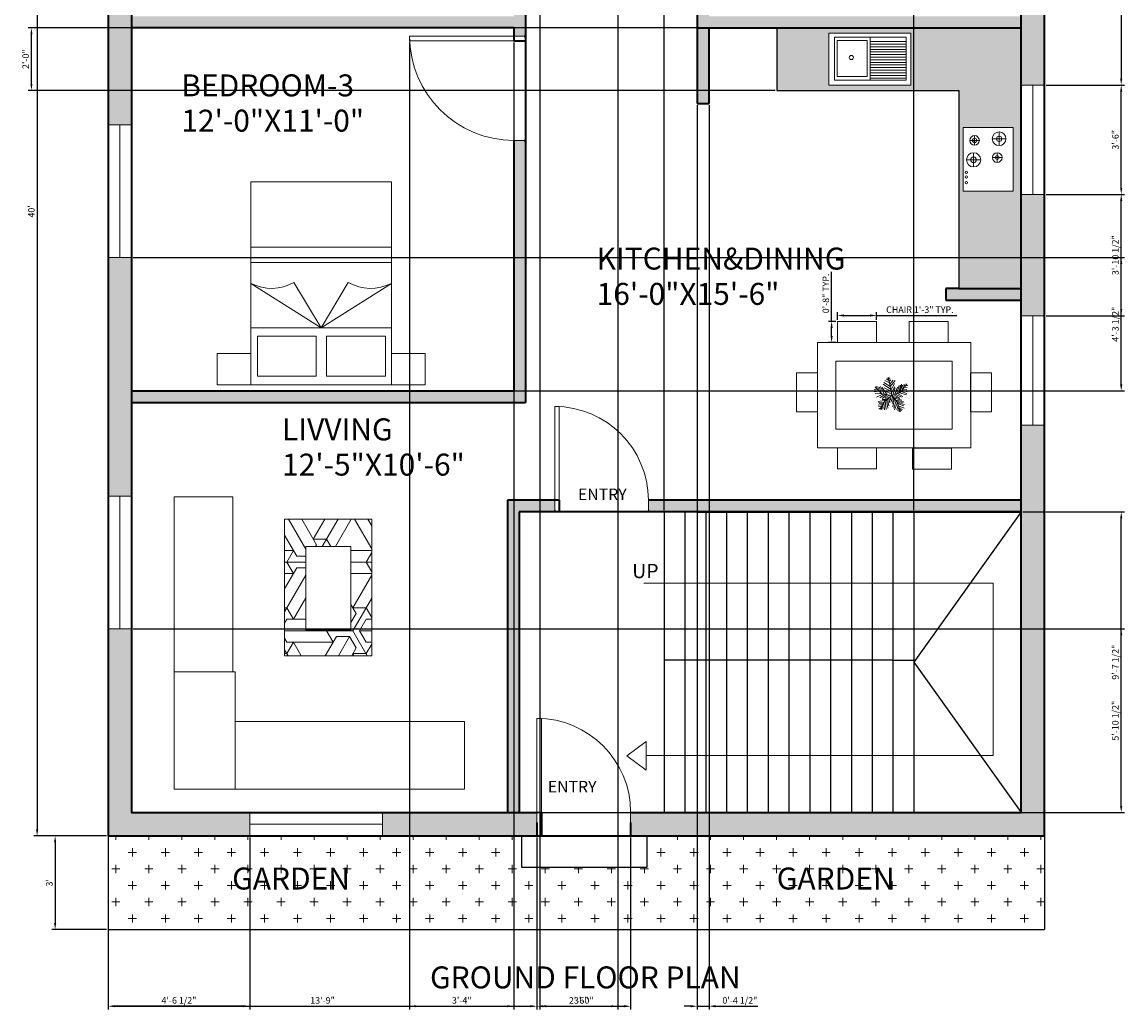
# Model space of a CAD drawing. Units: inches. Extents: x 10 to 434, y 91 to 681.
# Tile 1 of 2: x 10 to 434, y 91 to 471. Entities that reach past the tile are written whole.
import ezdxf

# ---------------------------------------------------------------- set-up
doc = ezdxf.new("R2010")
doc.units = ezdxf.units.IN
for name, color, linetype, lineweight in [('A-ANNO-DIMS', 2, 'Continuous', 18), ('A-ANNO-SYMB', 2, 'Continuous', 18), ('A-ANNO-TEXT', 7, 'Continuous', 18), ('A-AREA-IDEN', 7, 'Continuous', 18), ('A-DOOR', 4, 'Continuous', 18), ('A-EQPM', 8, 'Continuous', 18), ('A-FLOR-CASE', 8, 'Continuous', 25), ('A-FLOR-CASE-PATT', 141, 'Continuous', 13), ('A-FLOR-FIXT', 9, 'Continuous', 18), ('A-FLOR-FIXT-PATT', 9, 'Continuous', 13), ('A-FLOR-STRS', 7, 'Continuous', 25), ('A-FURN', 8, 'Continuous', 18), ('A-FURN-PATT', 8, 'Continuous', 13), ('A-GLAZ', 4, 'Continuous', 18), ('A-WALL', 7, 'Continuous', 35), ('A-WALL-PATT', 251, 'Continuous', 13), ('L-PLNT', 3, 'Continuous', 18), ('L-PLNT-BEDS', 3, 'Continuous', 25), ('L-PLNT-PATT', 114, 'Continuous', 13)]:
    doc.layers.add(name, color=color, linetype=linetype, lineweight=lineweight)
doc.styles.get("Standard").update_dxf_attribs({"font": 'arial.ttf'})
doc.dimstyles.new('ISO-25', dxfattribs={"dimtxt": 2.5, "dimasz": 2.5, "dimexe": 1.25, "dimexo": 0.625, "dimtad": 1, "dimlunit": 3, "dimtxsty": 'Standard', "dimcen": 2.5, "dimadec": 0, "dimazin": 0, "dimtfac": 1, "dimtmove": 0, "dimatfit": 3, "dimfxl": 1, "dimarcsym": 0})

# ---------------------------------------------------------------- blocks, each defined once
blk = doc.blocks.new('*U2')
for p, q in [((0, 0), (0, -4)), ((36, 0), (36, -4))]:
    blk.add_line(p, q)
blk.add_lwpolyline([(0, 0), (0, 36), (1.75, 36), (1.75, 0)], close=True)
blk.add_arc((0, 0), 36, 0, 90)
blk = doc.blocks.new('*U5')
for p, q in [((0, 0), (0, -4)), ((-40, 0), (-40, -4))]:
    blk.add_line(p, q)
blk.add_lwpolyline([(0, 0), (0, 40), (-1.75, 40), (-1.75, 0)], close=True)
blk.add_arc((0, 0), 40, 90, 180)
blk = doc.blocks.new('*U9')
for p, q in [((-3.665, 19.273), (-27.574, 35.527)), ((-5.114, 28.097), (-24.676, 40.636)), ((-7.288, 39.707), (-21.778, 46.673)), ((-8.737, 47.138), (-17.069, 52.711)), ((-10.186, 53.64), (-13.084, 55.962)), ((0, 0), (-10.5, 57)), ((-9.099, 51.782), (-6.563, 55.962)), ((-7.65, 43.423), (-2.578, 49.46)), ((-5.839, 35.992), (4.667, 48.067)), ((-5.114, 27.632), (10.463, 46.673)), ((-2.941, 16.486), (8.652, 37.85)), ((27, 9), (48, 36)), ((27.127, 9.056), (31.112, 35.992)), ((44.153, 36.456), (45.239, 32.741)), ((-47.498, 19.737), (-55.83, 18.344)), ((-40.615, 13.7), (-55.105, 10.913)), ((-31.5, 4.5), (-52.5, 25.5)), ((-33.37, 6.269), (-52.207, 5.34)), ((-48.585, 21.131), (-49.309, 29.026)), ((-28.299, 3.483), (-47.86, -5.805)), ((-43.513, 28.561), (-42.427, 15.558)), ((-38.442, 26.239), (-34.819, 7.663)), ((-21.416, 3.018), (-38.079, -8.128)), ((-35.544, 28.097), (-24.314, 3.947)), ((0, 0), (-31.5, 4.5)), ((-14.533, 2.09), (-30.834, 25.31)), ((-15.982, 2.09), (-30.11, -9.521)), ((-24.314, 23.917), (-2.941, 13.7)), ((0, 0), (-22.5, -19.5)), ((-6.563, 1.161), (-21.416, -8.128)), ((-20.691, 13.7), (-1.129, 4.876)), ((-1.129, 6.734), (9.014, 26.704)), ((0, 0), (27, 9)), ((0, 0), (18, -22.5)), ((3.942, 1.625), (11.187, 24.381)), ((6.478, 1.625), (26.04, -8.592)), ((10.101, 3.483), (17.708, 26.239)), ((11.187, 3.483), (30.749, -5.805)), ((16.259, 5.805), (23.142, 31.348)), ((18.07, 5.805), (35.096, -3.483)), ((22.055, 7.198), (27.489, 32.277)), ((24.229, 7.663), (46.688, 1.625)), ((29.662, 12.307), (48.137, 6.269)), ((31.836, 30.883), (32.561, 16.486)), ((33.285, 16.486), (48.862, 10.913)), ((35.096, 32.741), (37.27, 22.524)), ((36.183, 19.737), (48.137, 17.88)), ((38.719, 34.134), (41.979, 28.561)), ((40.53, 25.775), (48.862, 24.846)), ((43.791, 29.954), (51.036, 30.883)), ((-17.431, -15.094), (-42.789, -18.809)), ((-28.299, -29.026), (-42.789, -31.348)), ((-24.314, -21.596), (-42.427, -22.06)), ((-30.834, -34.135), (-42.427, -35.528)), ((-26.849, -26.24), (-40.253, -25.775)), ((-22.5, -19.5), (-37.5, -45)), ((-15.257, -12.772), (-30.11, -12.772)), ((-29.023, -30.884), (-27.936, -43.887)), ((-25.038, -23.918), (-22.865, -45.281)), ((-20.691, -18.345), (-17.793, -44.352)), ((-6.563, -5.805), (-19.967, -9.985)), ((-17.069, -15.094), (-12.721, -40.172)), ((-13.446, -11.378), (-8.737, -32.741)), ((-9.461, -8.592), (-6.201, -23.453)), ((-4.752, -3.483), (-3.665, -14.629)), ((2.493, -3.019), (-1.491, -20.202)), ((1.769, -2.555), (24.229, -9.521)), ((5.029, -6.27), (2.131, -25.775)), ((9.014, -11.378), (3.58, -35.992)), ((14.085, -16.951), (6.478, -40.172)), ((7.565, -9.056), (32.198, -14.629)), ((18.07, -22.524), (8.289, -45.745)), ((12.274, -15.094), (36.907, -18.809)), ((20.244, -30.419), (15.897, -44.816)), ((16.259, -19.738), (36.183, -22.989)), ((18, -22.5), (27, -52.5)), ((18.433, -22.524), (40.53, -29.026)), ((19.157, -25.311), (38.719, -33.206)), ((21.331, -32.741), (39.081, -40.636)), ((-34.457, -39.708), (-40.978, -42.494)), ((-32.646, -36.921), (-31.921, -44.352)), ((22.78, -37.85), (19.519, -48.532)), ((22.78, -38.314), (34.372, -44.816)), ((24.591, -45.745), (23.142, -50.854)), ((24.591, -43.423), (30.749, -47.603)), ((26.764, -49.925), (28.213, -50.854))]:
    blk.add_line(p, q)
blk = doc.blocks.new('*U10')
for p, q in [((0, 0), (0, -4)), ((36, 0), (36, -4))]:
    blk.add_line(p, q)
blk.add_lwpolyline([(0, 0), (0, 36), (1.75, 36), (1.75, 0)], close=True)
blk.add_arc((0, 0), 36, 0, 90)
blk = doc.blocks.new('*D11')
at = {"layer": 'A-ANNO-DIMS', "color": 0, "lineweight": -2, "transparency": 16777216}
for p, q in [((42.44, 638.74), (14.54, 638.74)), ((15.79, 636.24), (15.79, 161.24)), ((42.44, 158.74), (14.54, 158.74))]:
    blk.add_line(p, q, dxfattribs=at)
at = {"layer": 'A-ANNO-DIMS', "color": 0, "transparency": 16777216}
for points in [[(15.37, 636.24), (16.21, 636.24), (15.79, 638.74)], [(15.37, 161.24), (16.21, 161.24), (15.79, 158.74)]]:
    blk.add_solid(points, dxfattribs=at)
at = {"layer": 'Defpoints', "color": 0, "transparency": 16777216}
for p in [(43.07, 638.74), (15.79, 158.74), (43.07, 158.74)]:
    blk.add_point(p, dxfattribs=at)
at = {"layer": 'A-ANNO-DIMS', "color": 0, "transparency": 16777216, "insert": (13.89, 398.74), "char_height": 2.5, "attachment_point": 5, "rotation": 90}
blk.add_mtext("40'", dxfattribs=at)
blk = doc.blocks.new('*D13')
at = {"layer": 'A-ANNO-DIMS', "color": 0, "lineweight": -2, "transparency": 16777216}
for p, q in [((42.44, 158.74), (21.47, 158.74)), ((22.72, 156.24), (22.72, 125.24)), ((42.44, 122.74), (21.47, 122.74))]:
    blk.add_line(p, q, dxfattribs=at)
at = {"layer": 'A-ANNO-DIMS', "color": 0, "transparency": 16777216}
for points in [[(22.3, 156.24), (23.13, 156.24), (22.72, 158.74)], [(22.3, 125.24), (23.13, 125.24), (22.72, 122.74)]]:
    blk.add_solid(points, dxfattribs=at)
at = {"layer": 'Defpoints', "color": 0, "transparency": 16777216}
for p in [(43.07, 158.74), (22.72, 122.74), (43.07, 122.74)]:
    blk.add_point(p, dxfattribs=at)
at = {"layer": 'A-ANNO-DIMS', "color": 0, "transparency": 16777216, "insert": (20.81, 140.74), "char_height": 2.5, "attachment_point": 5, "rotation": 90}
blk.add_mtext("3'", dxfattribs=at)
blk = doc.blocks.new('BED-DOUBLE-WITH-NIGHTSTANDS')
for p, q in [((40, 21.85), (13, 39)), ((40, 21.85), (29.54, 39.37)), ((40, 21.85), (50.46, 39.37)), ((40, 21.85), (67, 39)), ((67, 21.85), (13, 21.85)), ((38.13, 3.34), (38.13, 18.76)), ((42.13, 3.34), (42.13, 18.76)), ((0, 0), (0, 12)), ((0, 12), (13, 12)), ((68, 12), (67, 12)), ((80, 12), (68, 12)), ((80, 0), (80, 12)), ((1, 0), (0, 0)), ((13, 0), (1, 0)), ((68, 0), (80, 0))]:
    blk.add_line(p, q)
for points in [[(67, 78), (13, 78), (13, 0), (67, 0)], [(67, 46.98), (13, 46.98), (13, 52.9), (67, 52.9)], [(67, 0), (68, 0), (68, 0), (67, 0)]]:
    blk.add_lwpolyline(points, close=True)
for points in [[(38.13, 3.34), (15.5, 3.34), (15.5, 18.76), (38.13, 18.76)], [(42.13, 18.76), (64.76, 18.76), (64.76, 3.34), (42.13, 3.34)]]:
    blk.add_lwpolyline(points)
for centre, start, end in [((20.93, 54.43), 242.8058, 299.7512), ((59.07, 54.43), 240.2488, 297.1942)]:
    blk.add_arc(centre, 17.35, start, end)
blk = doc.blocks.new('DINING-CHAIR')
blk.add_lwpolyline([(0, 0), (15.04, 0), (15.04, 8.09), (0, 8.09)], close=True)
blk = doc.blocks.new('WINDOW-51IN')
for p, q in [((0, 9), (0, 0)), ((51, 4.5), (51, 9)), ((51, 9), (51, 0)), ((0, 0), (0, 4.5)), ((0, 4.5), (51, 4.5))]:
    blk.add_line(p, q)
blk = doc.blocks.new('*D18')
at = {"layer": 'A-ANNO-DIMS', "color": 0, "lineweight": -2, "transparency": 16777216}
for p, q in [((323.44, 357.1), (323.44, 359.98)), ((325.94, 358.73), (335.98, 358.73)), ((338.48, 357.1), (338.48, 359.98)), ((338.48, 358.73), (369.27, 358.73))]:
    blk.add_line(p, q, dxfattribs=at)
at = {"layer": 'A-ANNO-DIMS', "color": 0, "transparency": 16777216}
for points in [[(325.94, 359.15), (325.94, 358.31), (323.44, 358.73)], [(335.98, 359.15), (335.98, 358.31), (338.48, 358.73)]]:
    blk.add_solid(points, dxfattribs=at)
at = {"layer": 'Defpoints', "color": 0, "transparency": 16777216}
for p in [(323.44, 356.47), (338.48, 358.73), (338.48, 356.47)]:
    blk.add_point(p, dxfattribs=at)
at = {"layer": 'A-ANNO-DIMS', "color": 0, "transparency": 16777216, "insert": (355.13, 360.65), "char_height": 2.5, "attachment_point": 5}
blk.add_mtext('CHAIR 1\'-3" TYP.', dxfattribs=at)
blk = doc.blocks.new('*D19')
at = {"layer": 'A-ANNO-DIMS', "color": 0, "lineweight": -2, "transparency": 16777216}
for p, q in [((321.19, 356.47), (321.19, 375.46)), ((322.82, 356.47), (319.94, 356.47)), ((321.19, 350.88), (321.19, 353.97)), ((322.82, 348.38), (319.94, 348.38))]:
    blk.add_line(p, q, dxfattribs=at)
at = {"layer": 'A-ANNO-DIMS', "color": 0, "transparency": 16777216}
for points in [[(320.77, 353.97), (321.6, 353.97), (321.19, 356.47)], [(320.77, 350.88), (321.6, 350.88), (321.19, 348.38)]]:
    blk.add_solid(points, dxfattribs=at)
at = {"layer": 'Defpoints', "color": 0, "transparency": 16777216}
for p in [(321.19, 356.47), (323.44, 356.47), (323.44, 348.38)]:
    blk.add_point(p, dxfattribs=at)
at = {"layer": 'A-ANNO-DIMS', "color": 0, "transparency": 16777216, "insert": (319.29, 367.22), "char_height": 2.5, "attachment_point": 5, "rotation": 90}
blk.add_mtext('0\'-8" TYP.', dxfattribs=at)
blk = doc.blocks.new('*D24')
at = {"layer": 'A-ANNO-DIMS', "color": 0, "lineweight": -2, "transparency": 16777216}
for p, q in [((43.07, 158.12), (43.07, 92.04)), ((207.93, 158.12), (207.93, 92.04)), ((45.57, 93.29), (205.43, 93.29))]:
    blk.add_line(p, q, dxfattribs=at)
at = {"layer": 'A-ANNO-DIMS', "color": 0, "transparency": 16777216}
for points in [[(45.57, 93.71), (45.57, 92.88), (43.07, 93.29)], [(205.43, 93.71), (205.43, 92.88), (207.93, 93.29)]]:
    blk.add_solid(points, dxfattribs=at)
at = {"layer": 'Defpoints', "color": 0, "transparency": 16777216}
for p in [(43.07, 158.74), (207.93, 158.74), (207.93, 93.29)]:
    blk.add_point(p, dxfattribs=at)
at = {"layer": 'A-ANNO-DIMS', "color": 0, "transparency": 16777216, "insert": (125.5, 95.2), "char_height": 2.5, "attachment_point": 5}
blk.add_mtext('13\'-9"', dxfattribs=at)
blk = doc.blocks.new('*D25')
at = {"layer": 'A-ANNO-DIMS', "color": 0, "lineweight": -2, "transparency": 16777216}
for p, q in [((207.93, 158.12), (207.93, 92.04)), ((243.93, 158.12), (243.93, 92.04)), ((210.43, 93.29), (241.43, 93.29))]:
    blk.add_line(p, q, dxfattribs=at)
at = {"layer": 'A-ANNO-DIMS', "color": 0, "transparency": 16777216}
for points in [[(210.43, 93.71), (210.43, 92.88), (207.93, 93.29)], [(241.43, 93.71), (241.43, 92.88), (243.93, 93.29)]]:
    blk.add_solid(points, dxfattribs=at)
at = {"layer": 'Defpoints', "color": 0, "transparency": 16777216}
for p in [(207.93, 158.74), (243.93, 158.74), (243.93, 93.29)]:
    blk.add_point(p, dxfattribs=at)
at = {"layer": 'A-ANNO-DIMS', "color": 0, "transparency": 16777216, "insert": (225.93, 95.2), "char_height": 2.5, "attachment_point": 5}
blk.add_mtext('3\'-0"', dxfattribs=at)
blk = doc.blocks.new('*D26')
at = {"layer": 'A-ANNO-DIMS', "color": 0, "lineweight": -2, "transparency": 16777216}
for p, q in [((394.69, 283.24), (433.77, 283.24)), ((432.52, 170.24), (432.52, 280.74)), ((394.69, 167.74), (433.77, 167.74))]:
    blk.add_line(p, q, dxfattribs=at)
at = {"layer": 'A-ANNO-DIMS', "color": 0, "transparency": 16777216}
for points in [[(432.1, 280.74), (432.93, 280.74), (432.52, 283.24)], [(432.1, 170.24), (432.93, 170.24), (432.52, 167.74)]]:
    blk.add_solid(points, dxfattribs=at)
at = {"layer": 'Defpoints', "color": 0, "transparency": 16777216}
for p in [(394.07, 283.24), (432.52, 283.24), (394.07, 167.74)]:
    blk.add_point(p, dxfattribs=at)
at = {"layer": 'A-ANNO-DIMS', "color": 0, "transparency": 16777216, "insert": (430.6, 225.49), "char_height": 2.5, "attachment_point": 5, "rotation": 90}
blk.add_mtext('9\'-7 1/2"', dxfattribs=at)
blk = doc.blocks.new('*D27')
at = {"layer": 'A-ANNO-DIMS', "color": 0, "lineweight": -2, "transparency": 16777216}
for p, q in [((352.79, 283.87), (352.79, 669.44)), ((355.29, 668.19), (391.57, 668.19)), ((394.07, 283.87), (394.07, 669.44))]:
    blk.add_line(p, q, dxfattribs=at)
at = {"layer": 'A-ANNO-DIMS', "color": 0, "transparency": 16777216}
for points in [[(355.29, 668.61), (355.29, 667.78), (352.79, 668.19)], [(391.57, 668.61), (391.57, 667.78), (394.07, 668.19)]]:
    blk.add_solid(points, dxfattribs=at)
at = {"layer": 'Defpoints', "color": 0, "transparency": 16777216}
for p in [(394.07, 668.19), (352.79, 283.24), (394.07, 283.24)]:
    blk.add_point(p, dxfattribs=at)
at = {"layer": 'A-ANNO-DIMS', "color": 0, "transparency": 16777216, "insert": (373.43, 670.11), "char_height": 2.5, "attachment_point": 5}
blk.add_mtext('3\'-5 1/2"', dxfattribs=at)
blk = doc.blocks.new('*D28')
at = {"layer": 'A-ANNO-DIMS', "color": 0, "lineweight": -2, "transparency": 16777216}
for p, q in [((256.79, 283.87), (256.79, 669.44)), ((259.29, 668.19), (350.29, 668.19)), ((352.79, 283.87), (352.79, 669.44))]:
    blk.add_line(p, q, dxfattribs=at)
at = {"layer": 'A-ANNO-DIMS', "color": 0, "transparency": 16777216}
for points in [[(259.29, 668.61), (259.29, 667.78), (256.79, 668.19)], [(350.29, 668.61), (350.29, 667.78), (352.79, 668.19)]]:
    blk.add_solid(points, dxfattribs=at)
at = {"layer": 'Defpoints', "color": 0, "transparency": 16777216}
for p in [(352.79, 668.19), (256.79, 283.24), (352.79, 283.24)]:
    blk.add_point(p, dxfattribs=at)
at = {"layer": 'A-ANNO-DIMS', "color": 0, "transparency": 16777216, "insert": (304.79, 670.1), "char_height": 2.5, "attachment_point": 5}
blk.add_mtext('8\'-0"', dxfattribs=at)
blk = doc.blocks.new('*D32')
at = {"layer": 'A-ANNO-DIMS', "color": 0, "lineweight": -2, "transparency": 16777216}
for p, q in [((52.69, 238.26), (433.77, 238.26)), ((432.52, 170.24), (432.52, 235.76)), ((52.69, 167.74), (433.77, 167.74))]:
    blk.add_line(p, q, dxfattribs=at)
at = {"layer": 'A-ANNO-DIMS', "color": 0, "transparency": 16777216}
for points in [[(432.1, 235.76), (432.93, 235.76), (432.52, 238.26)], [(432.1, 170.24), (432.93, 170.24), (432.52, 167.74)]]:
    blk.add_solid(points, dxfattribs=at)
at = {"layer": 'Defpoints', "color": 0, "transparency": 16777216}
for p in [(52.07, 238.26), (432.52, 238.26), (52.07, 167.74)]:
    blk.add_point(p, dxfattribs=at)
at = {"layer": 'A-ANNO-DIMS', "color": 0, "transparency": 16777216, "insert": (430.6, 203), "char_height": 2.5, "attachment_point": 5, "rotation": 90}
blk.add_mtext('5\'-10 1/2"', dxfattribs=at)
blk = doc.blocks.new('*D33')
at = {"layer": 'A-ANNO-DIMS', "color": 0, "lineweight": -2, "transparency": 16777216}
for p, q in [((52.69, 381.02), (433.77, 381.02)), ((432.52, 332.24), (432.52, 378.52)), ((52.69, 329.74), (433.77, 329.74))]:
    blk.add_line(p, q, dxfattribs=at)
at = {"layer": 'A-ANNO-DIMS', "color": 0, "transparency": 16777216}
for points in [[(432.1, 378.52), (432.93, 378.52), (432.52, 381.02)], [(432.1, 332.24), (432.93, 332.24), (432.52, 329.74)]]:
    blk.add_solid(points, dxfattribs=at)
at = {"layer": 'Defpoints', "color": 0, "transparency": 16777216}
for p in [(52.07, 381.02), (432.52, 381.02), (52.07, 329.74)]:
    blk.add_point(p, dxfattribs=at)
at = {"layer": 'A-ANNO-DIMS', "color": 0, "transparency": 16777216, "insert": (430.6, 355.38), "char_height": 2.5, "attachment_point": 5, "rotation": 90}
blk.add_mtext('4\'-3 1/2"', dxfattribs=at)
blk = doc.blocks.new('*D36')
at = {"layer": 'A-ANNO-DIMS', "color": 0, "lineweight": -2, "transparency": 16777216}
for p, q in [((403.69, 544.74), (433.77, 544.74)), ((432.52, 542.24), (432.52, 449.76)), ((403.69, 447.26), (433.77, 447.26))]:
    blk.add_line(p, q, dxfattribs=at)
at = {"layer": 'A-ANNO-DIMS', "color": 0, "transparency": 16777216}
for points in [[(432.1, 542.24), (432.93, 542.24), (432.52, 544.74)], [(432.1, 449.76), (432.93, 449.76), (432.52, 447.26)]]:
    blk.add_solid(points, dxfattribs=at)
at = {"layer": 'Defpoints', "color": 0, "transparency": 16777216}
for p in [(403.07, 544.74), (403.07, 447.26), (432.52, 447.26)]:
    blk.add_point(p, dxfattribs=at)
at = {"layer": 'A-ANNO-DIMS', "color": 0, "transparency": 16777216, "insert": (430.6, 496), "char_height": 2.5, "attachment_point": 5, "rotation": 90}
blk.add_mtext('8\'-1 1/2"', dxfattribs=at)
blk = doc.blocks.new('*D37')
at = {"layer": 'A-ANNO-DIMS', "color": 0, "lineweight": -2, "transparency": 16777216}
for p, q in [((403.69, 447.26), (433.77, 447.26)), ((432.52, 407.76), (432.52, 444.76)), ((403.69, 405.26), (433.77, 405.26))]:
    blk.add_line(p, q, dxfattribs=at)
at = {"layer": 'A-ANNO-DIMS', "color": 0, "transparency": 16777216}
for points in [[(432.1, 444.76), (432.93, 444.76), (432.52, 447.26)], [(432.1, 407.76), (432.93, 407.76), (432.52, 405.26)]]:
    blk.add_solid(points, dxfattribs=at)
at = {"layer": 'Defpoints', "color": 0, "transparency": 16777216}
for p in [(403.07, 447.26), (432.52, 447.26), (403.07, 405.26)]:
    blk.add_point(p, dxfattribs=at)
at = {"layer": 'A-ANNO-DIMS', "color": 0, "transparency": 16777216, "insert": (430.61, 426.26), "char_height": 2.5, "attachment_point": 5, "rotation": 90}
blk.add_mtext('3\'-6"', dxfattribs=at)
blk = doc.blocks.new('*D38')
at = {"layer": 'A-ANNO-DIMS', "color": 0, "lineweight": -2, "transparency": 16777216}
for p, q in [((403.69, 405.26), (433.77, 405.26)), ((432.52, 361.08), (432.52, 402.76)), ((403.69, 358.58), (433.77, 358.58))]:
    blk.add_line(p, q, dxfattribs=at)
at = {"layer": 'A-ANNO-DIMS', "color": 0, "transparency": 16777216}
for points in [[(432.1, 402.76), (432.93, 402.76), (432.52, 405.26)], [(432.1, 361.08), (432.93, 361.08), (432.52, 358.58)]]:
    blk.add_solid(points, dxfattribs=at)
at = {"layer": 'Defpoints', "color": 0, "transparency": 16777216}
for p in [(403.07, 405.26), (432.52, 405.26), (403.07, 358.58)]:
    blk.add_point(p, dxfattribs=at)
at = {"layer": 'A-ANNO-DIMS', "color": 0, "transparency": 16777216, "insert": (430.6, 381.92), "char_height": 2.5, "attachment_point": 5, "rotation": 90}
blk.add_mtext('3\'-10 1/2"', dxfattribs=at)
blk = doc.blocks.new('*D39')
at = {"layer": 'A-ANNO-DIMS', "color": 0, "lineweight": -2, "transparency": 16777216}
for p, q in [((43.07, 158.12), (43.07, 92.04)), ((97.57, 158.12), (97.57, 92.04)), ((95.07, 93.29), (45.57, 93.29))]:
    blk.add_line(p, q, dxfattribs=at)
at = {"layer": 'A-ANNO-DIMS', "color": 0, "transparency": 16777216}
for points in [[(45.57, 93.71), (45.57, 92.88), (43.07, 93.29)], [(95.07, 93.71), (95.07, 92.88), (97.57, 93.29)]]:
    blk.add_solid(points, dxfattribs=at)
at = {"layer": 'Defpoints', "color": 0, "transparency": 16777216}
for p in [(43.07, 158.74), (97.57, 158.74), (43.07, 93.29)]:
    blk.add_point(p, dxfattribs=at)
at = {"layer": 'A-ANNO-DIMS', "color": 0, "transparency": 16777216, "insert": (70.32, 95.21), "char_height": 2.5, "attachment_point": 5}
blk.add_mtext('4\'-6 1/2"', dxfattribs=at)
blk = doc.blocks.new('*D40')
at = {"layer": 'A-ANNO-DIMS', "color": 0, "lineweight": -2, "transparency": 16777216}
for p, q in [((208.98, 533.52), (208.98, 92.04)), ((238.98, 533.12), (238.98, 92.04)), ((211.48, 93.29), (236.48, 93.29))]:
    blk.add_line(p, q, dxfattribs=at)
at = {"layer": 'A-ANNO-DIMS', "color": 0, "transparency": 16777216}
for points in [[(211.48, 93.71), (211.48, 92.88), (208.98, 93.29)], [(236.48, 93.71), (236.48, 92.88), (238.98, 93.29)]]:
    blk.add_solid(points, dxfattribs=at)
at = {"layer": 'Defpoints', "color": 0, "transparency": 16777216}
for p in [(208.98, 534.14), (238.98, 533.74), (238.98, 93.29)]:
    blk.add_point(p, dxfattribs=at)
at = {"layer": 'A-ANNO-DIMS', "color": 0, "transparency": 16777216, "insert": (223.98, 95.2), "char_height": 2.5, "attachment_point": 5}
blk.add_mtext('2\'-6"', dxfattribs=at)
blk = doc.blocks.new('*D41')
at = {"layer": 'A-ANNO-DIMS', "color": 0, "lineweight": -2, "transparency": 16777216}
for p, q in [((158.99, 463.66), (158.99, 92.04)), ((199.07, 463.66), (199.07, 92.04)), ((161.49, 93.29), (196.57, 93.29))]:
    blk.add_line(p, q, dxfattribs=at)
at = {"layer": 'A-ANNO-DIMS', "color": 0, "transparency": 16777216}
for points in [[(161.49, 93.71), (161.49, 92.88), (158.99, 93.29)], [(196.57, 93.71), (196.57, 92.88), (199.07, 93.29)]]:
    blk.add_solid(points, dxfattribs=at)
at = {"layer": 'Defpoints', "color": 0, "transparency": 16777216}
for p in [(158.99, 464.29), (199.07, 464.29), (199.07, 93.29)]:
    blk.add_point(p, dxfattribs=at)
at = {"layer": 'A-ANNO-DIMS', "color": 0, "transparency": 16777216, "insert": (179.03, 95.2), "char_height": 2.5, "attachment_point": 5}
blk.add_mtext('3\'-4"', dxfattribs=at)
blk = doc.blocks.new('*D42')
at = {"layer": 'A-ANNO-DIMS', "color": 0, "lineweight": -2, "transparency": 16777216}
for p, q in [((299.46, 469.24), (12.37, 469.24)), ((13.62, 447.74), (13.62, 466.74)), ((299.46, 445.24), (12.37, 445.24))]:
    blk.add_line(p, q, dxfattribs=at)
at = {"layer": 'A-ANNO-DIMS', "color": 0, "transparency": 16777216}
for points in [[(13.2, 466.74), (14.03, 466.74), (13.62, 469.24)], [(13.2, 447.74), (14.03, 447.74), (13.62, 445.24)]]:
    blk.add_solid(points, dxfattribs=at)
at = {"layer": 'Defpoints', "color": 0, "transparency": 16777216}
for p in [(13.62, 469.24), (300.08, 469.24), (300.08, 445.24)]:
    blk.add_point(p, dxfattribs=at)
at = {"layer": 'A-ANNO-DIMS', "color": 0, "transparency": 16777216, "insert": (11.71, 457.24), "char_height": 2.5, "attachment_point": 5, "rotation": 90}
blk.add_mtext('2\'-0"', dxfattribs=at)
blk = doc.blocks.new('*D43')
at = {"layer": 'A-ANNO-DIMS', "color": 0, "lineweight": -2, "transparency": 16777216}
for p, q in [((269.57, 439.62), (269.57, 92.04)), ((274.07, 439.62), (274.07, 92.04)), ((267.07, 93.29), (264.57, 93.29)), ((269.57, 93.29), (274.07, 93.29)), ((276.57, 93.29), (292.79, 93.29))]:
    blk.add_line(p, q, dxfattribs=at)
at = {"layer": 'A-ANNO-DIMS', "color": 0, "transparency": 16777216}
for points in [[(267.07, 93.71), (267.07, 92.88), (269.57, 93.29)], [(276.57, 93.71), (276.57, 92.88), (274.07, 93.29)]]:
    blk.add_solid(points, dxfattribs=at)
at = {"layer": 'Defpoints', "color": 0, "transparency": 16777216}
for p in [(269.57, 440.24), (274.07, 440.24), (274.07, 93.29)]:
    blk.add_point(p, dxfattribs=at)
at = {"layer": 'A-ANNO-DIMS', "color": 0, "transparency": 16777216, "insert": (285.93, 95.21), "char_height": 2.5, "attachment_point": 5}
blk.add_mtext('0\'-4 1/2"', dxfattribs=at)

msp = doc.modelspace()

# ---------------------------------------------------------------- hatches: boundary and pattern name
at = {"layer": 'A-FLOR-CASE-PATT'}
h = msp.add_hatch(color=256, dxfattribs=at)
h.dxf.hatch_style = 1
h.paths.add_polyline_path([(394.066, 469.244), (300.082, 469.244), (300.082, 445.244), (370.066, 445.244), (370.066, 369.085), (394.066, 369.085)])
h.paths.add_polyline_path([(351.692, 447.254), (320.159, 447.254), (320.159, 467.243), (351.692, 467.243)], flags=16)
h.paths.add_polyline_path([(349.81, 449.213), (322.277, 449.213), (322.277, 465.675), (349.81, 465.675)], flags=0)
h.paths.add_polyline_path([(334.86, 450.587), (323.321, 450.587), (323.321, 464.376), (334.86, 464.376)], flags=0)
h.paths.add_polyline_path([(327.986, 457.898, -1), (329.557, 457.898, -1)], flags=0)
h.paths.add_polyline_path([(371.798, 430.985), (390.936, 430.985), (390.936, 406.486), (371.798, 406.486)], flags=16)
h.paths.add_polyline_path([(377.994, 426.018, -1), (374.301, 426.018, -1)], flags=0)
h.paths.add_polyline_path([(376.99, 426.018, -1), (375.305, 426.018, -1)], flags=0)
h.paths.add_polyline_path([(388.213, 426.639, -1), (382.972, 426.639, -1)], flags=0)
h.paths.add_polyline_path([(386.615, 426.639, -1), (384.57, 426.639, -1)], flags=0)
h.paths.add_polyline_path([(378.499, 418.566, -1), (373.05, 418.566, -1)], flags=0)
h.paths.add_polyline_path([(376.878, 418.566, -1), (374.671, 418.566, -1)], flags=0)
h.paths.add_polyline_path([(386.71, 419.436, -1), (382.984, 419.436, -1)], flags=0)
h.paths.add_polyline_path([(385.57, 419.436, -1), (384.123, 419.436, -1)], flags=0)
h.paths.add_polyline_path([(373.459, 413.765, -1), (372.584, 413.765, -1)], flags=0)
h.paths.add_polyline_path([(373.459, 411.997, -1), (372.584, 411.997, -1)], flags=0)
h.paths.add_polyline_path([(373.459, 409.761, -1), (372.584, 409.761, -1)], flags=0)
at = {"layer": 'A-FLOR-FIXT-PATT'}
h = msp.add_hatch(dxfattribs=at)
h.set_pattern_fill('ANSI31', color=256, scale=0.314961, angle=-45, style=0)
h.paths.add_polyline_path([(336.043, 449.801), (349.81, 449.801), (349.81, 464.801), (336.043, 464.801)])
at = {"layer": 'A-FURN-PATT'}
h = msp.add_hatch(dxfattribs=at)
h.set_pattern_fill('ESCHER', color=256)
h.paths.add_polyline_path([(136.437, 269.899), (119.058, 269.899), (119.058, 237.78), (136.437, 237.78)], flags=0)
h.paths.add_polyline_path([(144.395, 280.467), (110.907, 280.467), (110.907, 227.986), (144.395, 227.986)])
h.paths.add_polyline_path([(119.058, 237.78), (119.058, 269.899), (136.437, 269.899), (136.437, 237.78)], flags=16)
at = {"layer": 'A-WALL-PATT'}
h = msp.add_hatch(color=256, dxfattribs=at)
h.dxf.hatch_style = 1
h.paths.add_polyline_path([(84.716, 634.244), (84.716, 638.744), (43.066, 638.744), (43.066, 588.73), (47.566, 588.73), (52.066, 588.73), (52.066, 629.744), (84.716, 629.744)])
h.paths.add_polyline_path([(227.044, 638.744), (135.716, 638.744), (135.716, 629.744), (227.044, 629.744)])
h.paths.add_polyline_path([(52.066, 537.73), (43.066, 537.73), (43.066, 432.018), (52.066, 432.018)])
h.paths.add_polyline_path([(52.066, 381.018), (43.066, 381.018), (43.066, 289.264), (47.566, 289.264), (52.066, 289.264)])
h.paths.add_polyline_path([(52.066, 238.264), (43.066, 238.264), (43.066, 158.744), (97.573, 158.744), (97.573, 163.244), (97.573, 167.744), (52.066, 167.744)])
h.paths.add_polyline_path([(207.929, 163.896), (207.929, 167.744), (148.573, 167.744), (148.573, 158.744), (207.929, 158.744)])
h.paths.add_polyline_path([(403.066, 316.579), (394.066, 316.579), (394.066, 167.744), (243.929, 167.744), (243.929, 163.896), (243.929, 158.744), (403.066, 158.744)])
h.paths.add_polyline_path([(403.066, 405.259), (398.566, 405.259), (394.066, 405.259), (394.066, 358.579), (403.066, 358.579)])
h.paths.add_polyline_path([(394.066, 473.744), (274.066, 473.744), (274.066, 476.846), (270.089, 476.846), (269.566, 476.846), (269.566, 469.244), (394.066, 469.244)])
h.paths.add_polyline_path([(203.566, 475.661), (203.066, 475.661), (199.066, 475.661), (199.066, 473.744), (52.066, 473.744), (52.066, 469.244), (199.066, 469.244), (199.066, 466.04), (202.989, 466.04), (203.566, 466.04), (203.566, 469.244)])
h.paths.add_polyline_path([(203.566, 426.04), (202.989, 426.04), (199.066, 426.04), (199.066, 329.744), (184.066, 329.744), (52.066, 329.744), (52.066, 325.244), (184.066, 325.244), (203.566, 325.244)])
h.paths.add_polyline_path([(201.066, 283.244), (202.066, 283.244), (214.742, 283.244), (214.742, 283.768), (214.742, 287.744), (202.066, 287.744), (196.566, 287.744), (196.566, 167.744), (201.066, 167.744)])
h.paths.add_polyline_path([(394.066, 287.744), (250.742, 287.744), (250.742, 283.768), (250.742, 283.244), (394.066, 283.244)], flags=17)
h.paths.add_polyline_path([(394.066, 369.085), (370.066, 369.085), (365.066, 369.085), (365.066, 364.585), (394.066, 364.585)])
h.paths.add_polyline_path([(274.066, 469.244), (269.566, 469.244), (269.566, 440.244), (274.066, 440.244)])
h.paths.add_polyline_path([(403.066, 544.736), (394.066, 544.736), (394.066, 447.259), (403.066, 447.259)])
h.paths.add_polyline_path([(206.394, 574.303), (265.532, 574.303), (265.532, 587.233), (206.394, 587.233)], flags=9)
h.paths.add_polyline_path([(206.366, 587.835), (252.012, 587.835), (252.012, 600.937), (206.366, 600.937)], flags=9)
h.paths.add_polyline_path([(303.038, 504.495), (375.295, 504.495), (375.295, 517.433), (303.038, 517.433)], flags=9)
h.paths.add_polyline_path([(303.011, 518.033), (378.795, 518.033), (378.795, 531.136), (303.011, 531.136)], flags=9)
at = {"layer": 'L-PLNT-PATT'}
h = msp.add_hatch(dxfattribs=at)
h.set_pattern_fill('CROSS', color=256)
h.paths.add_polyline_path([(403.066, 158.744), (250.331, 158.744), (250.331, 146.744), (201.93, 146.744), (201.93, 158.744), (43.066, 158.744), (43.066, 122.744), (403.066, 122.744)])
h.paths.add_polyline_path([(297.922, 135.815), (352.738, 135.815), (352.738, 148.909), (297.922, 148.909)], flags=24)
h.paths.add_polyline_path([(88.587, 135.815), (143.403, 135.815), (143.403, 148.909), (88.587, 148.909)], flags=24)

# ---------------------------------------------------------------- linework, layer by layer
at = {"layer": 'A-ANNO-SYMB'}
for p, q in [((249.07, 255.919), (383.252, 255.919)), ((383.252, 255.919), (383.252, 189.698)), ((242.461, 189.525), (249.937, 194.967)), ((249.937, 189.698), (249.937, 194.967)), ((249.937, 194.967), (249.937, 183.991)), ((249.937, 183.991), (242.461, 189.525)), ((383.252, 189.698), (249.937, 189.698))]:
    msp.add_line(p, q, dxfattribs=at)
at = {"layer": 'A-EQPM'}
for p, q in [((385.592, 424.018), (385.592, 429.259)), ((374.301, 426.018), (377.994, 426.018)), ((376.147, 424.171), (376.147, 427.865)), ((382.972, 426.639), (388.213, 426.639)), ((375.775, 415.842), (375.775, 421.291)), ((384.847, 420.159), (384.847, 421.298)), ((384.847, 418.154), (384.847, 420.159)), ((373.05, 418.566), (378.499, 418.566)), ((382.984, 419.436), (386.71, 419.436)), ((384.847, 417.573), (384.847, 418.712))]:
    msp.add_line(p, q, dxfattribs=at)
msp.add_lwpolyline([(371.798, 430.985), (390.936, 430.985), (390.936, 406.486), (371.798, 406.486)], close=True, dxfattribs=at)
for centre, radius in [((385.592, 426.639), 2.62), ((376.147, 426.018), 1.847), ((376.147, 426.018), 0.843), ((385.592, 426.639), 1.022), ((375.775, 418.566), 2.725), ((384.847, 419.436), 1.863), ((384.847, 419.436), 0.724), ((375.775, 418.566), 1.104), ((373.022, 413.765), 0.437), ((373.022, 411.997), 0.437), ((373.022, 409.761), 0.437)]:
    msp.add_circle(centre, radius, dxfattribs=at)
at = {"layer": 'A-FLOR-CASE'}
for p, q in [((300.082, 469.244), (300.082, 445.244)), ((300.082, 445.244), (370.066, 445.244)), ((370.066, 445.244), (370.066, 369.085))]:
    msp.add_line(p, q, dxfattribs=at)
at = {"layer": 'A-FLOR-FIXT'}
msp.add_line((336.043, 465.675), (336.043, 449.213), dxfattribs=at)
for points in [[(320.159, 467.243), (351.692, 467.243), (351.692, 447.254), (320.159, 447.254)], [(322.277, 465.675), (349.81, 465.675), (349.81, 449.213), (322.277, 449.213)], [(323.321, 464.376), (334.86, 464.376), (334.86, 450.587), (323.321, 450.587)]]:
    msp.add_lwpolyline(points, close=True, dxfattribs=at)
msp.add_circle((328.771, 457.898), 0.786, dxfattribs=at)
at = {"layer": 'A-FLOR-STRS'}
for p, q in [((256.787, 283.244), (256.787, 226.244)), ((264.787, 283.244), (264.787, 226.244)), ((272.787, 283.244), (272.787, 226.244)), ((280.787, 283.244), (280.787, 226.244)), ((288.787, 283.244), (288.787, 226.244)), ((296.787, 283.244), (296.787, 226.244)), ((304.787, 283.244), (304.787, 226.244)), ((312.787, 283.244), (312.787, 226.244)), ((320.787, 283.244), (320.787, 226.244)), ((328.787, 283.244), (328.787, 226.244)), ((336.787, 283.244), (336.787, 226.244)), ((352.787, 283.244), (344.787, 283.244)), ((344.787, 283.244), (344.787, 226.244)), ((352.787, 283.244), (352.787, 167.744)), ((394.066, 283.244), (352.787, 225.494)), ((344.787, 226.244), (256.787, 226.244)), ((256.787, 226.244), (256.787, 167.744)), ((264.787, 226.244), (264.787, 167.744)), ((272.787, 226.244), (272.787, 167.744)), ((280.787, 226.244), (280.787, 167.744)), ((288.787, 226.244), (288.787, 167.744)), ((296.787, 226.244), (296.787, 167.744)), ((304.787, 226.244), (304.787, 167.744)), ((312.787, 226.244), (312.787, 167.744)), ((320.787, 226.244), (320.787, 167.744)), ((328.787, 226.244), (328.787, 167.744)), ((336.787, 226.244), (336.787, 167.744)), ((344.787, 226.244), (344.787, 167.744)), ((344.787, 226.244), (352.787, 226.244)), ((352.787, 225.494), (394.066, 167.744)), ((201.93, 158.744), (201.93, 146.744)), ((250.331, 146.744), (250.331, 158.744)), ((201.93, 146.744), (250.331, 146.744))]:
    msp.add_line(p, q, dxfattribs=at)
at = {"layer": 'A-FURN'}
for points in [[(315.732, 348.383), (374.719, 348.383), (374.719, 307.929), (315.732, 307.929)], [(322.877, 341.238), (367.574, 341.238), (367.574, 315.074), (322.877, 315.074)], [(68.472, 221.807), (91.068, 221.807), (91.068, 288.996), (68.472, 288.996)], [(110.907, 280.467), (144.395, 280.467), (144.395, 227.986), (110.907, 227.986)], [(119.058, 269.899), (136.437, 269.899), (136.437, 237.78), (119.058, 237.78)], [(68.472, 221.807), (91.863, 221.807), (91.863, 176.685), (68.472, 176.685)], [(91.863, 176.685), (180.113, 176.685), (180.113, 202.752), (91.863, 202.752)]]:
    msp.add_lwpolyline(points, close=True, dxfattribs=at)
at = {"layer": 'A-GLAZ'}
for p, q in [((398.566, 447.259), (394.066, 447.259)), ((394.066, 447.259), (403.066, 447.259)), ((398.566, 405.259), (398.566, 447.259)), ((43.066, 432.018), (52.066, 432.018)), ((52.066, 432.018), (47.566, 432.018)), ((47.566, 432.018), (47.566, 381.018)), ((394.066, 405.259), (403.066, 405.259)), ((403.066, 405.259), (398.566, 405.259)), ((52.066, 381.018), (43.066, 381.018)), ((47.566, 381.018), (52.066, 381.018)), ((398.566, 358.579), (394.066, 358.579)), ((394.066, 358.579), (403.066, 358.579)), ((398.566, 316.579), (398.566, 358.579)), ((394.066, 316.579), (403.066, 316.579))]:
    msp.add_line(p, q, dxfattribs=at)
at = {"layer": 'A-WALL'}
for p, q in [((203.566, 533.744), (203.566, 469.244)), ((269.566, 533.744), (269.566, 469.244)), ((199.066, 469.244), (52.066, 469.244)), ((52.066, 469.244), (52.066, 337.244)), ((52.066, 469.244), (52.066, 325.244)), ((199.066, 469.244), (199.066, 464.29)), ((203.566, 469.244), (203.566, 325.244)), ((269.566, 469.244), (394.066, 469.244)), ((269.566, 469.244), (269.566, 440.244)), ((274.066, 440.244), (274.066, 469.244)), ((198.989, 464.29), (203.566, 464.29)), ((202.989, 466.04), (203.566, 466.04)), ((269.566, 440.244), (274.066, 440.244)), ((199.066, 426.04), (199.066, 329.744)), ((202.989, 426.04), (203.566, 426.04)), ((370.066, 369.085), (365.066, 369.085)), ((365.066, 369.085), (365.066, 364.585)), ((370.066, 369.085), (394.066, 369.085)), ((365.066, 364.585), (394.066, 364.585)), ((52.066, 329.744), (184.066, 329.744)), ((184.066, 329.744), (199.066, 329.744)), ((52.066, 325.244), (184.066, 325.244)), ((52.066, 325.244), (52.066, 167.744)), ((184.066, 325.244), (203.566, 325.244)), ((196.566, 287.744), (196.566, 167.744)), ((202.066, 287.744), (196.566, 287.744)), ((216.492, 287.744), (202.066, 287.744)), ((216.492, 287.768), (216.492, 283.244)), ((394.066, 287.744), (250.742, 287.744)), ((201.066, 283.244), (201.066, 167.744)), ((202.066, 283.244), (201.066, 283.244)), ((394.066, 283.244), (202.066, 283.244)), ((214.742, 283.768), (214.742, 283.244)), ((250.742, 283.768), (250.742, 283.244)), ((269.566, 283.244), (394.066, 283.244)), ((209.679, 167.896), (209.679, 158.744)), ((207.929, 163.896), (207.929, 158.744)), ((243.929, 163.896), (243.929, 158.744))]:
    msp.add_line(p, q, dxfattribs=at)
msp.add_lwpolyline([(43.066, 158.744), (403.066, 158.744), (403.066, 638.744), (43.066, 638.744)], close=True, dxfattribs=at)
msp.add_lwpolyline([(243.929, 167.744), (394.066, 167.744), (394.066, 629.744), (52.066, 629.744), (52.066, 167.744), (207.929, 167.744)], dxfattribs=at)
at = {"layer": 'L-PLNT-BEDS'}
for p, q in [((43.066, 158.744), (43.066, 122.744)), ((403.066, 158.744), (403.066, 122.744)), ((43.066, 122.744), (403.066, 122.744))]:
    msp.add_line(p, q, dxfattribs=at)

# ---------------------------------------------------------------- block references
at = {"layer": 'A-DOOR', "rotation": 90}
msp.add_blockref('*U5', (198.989, 466.04), dxfattribs=at)
at = {"layer": 'A-DOOR'}
for name, p in [('*U2', (214.742, 287.768)), ('*U10', (207.929, 167.896))]:
    msp.add_blockref(name, p, dxfattribs=at)
at = {"layer": 'A-FURN'}
for name, p in [('BED-DOUBLE-WITH-NIGHTSTANDS', (84.952, 332.088)), ('DINING-CHAIR', (323.442, 348.383)), ('DINING-CHAIR', (350.944, 348.383)), ('DINING-CHAIR', (323.442, 299.841)), ('DINING-CHAIR', (352.264, 299.721))]:
    msp.add_blockref(name, p, dxfattribs=at)
for p, rotation in [((315.732, 321.65), 90.00000000000142), ((382.638, 321.65), 90.00000000000087)]:
    msp.add_blockref('DINING-CHAIR', p, dxfattribs=dict(at, rotation=rotation))
at = {"layer": 'A-GLAZ'}
for p, rotation in [((52.065, 238.265), 90.0000000000003), ((148.573, 167.743), 180)]:
    msp.add_blockref('WINDOW-51IN', p, dxfattribs=dict(at, rotation=rotation))
at = {"layer": 'L-PLNT', "xscale": 0.121493366931729, "yscale": 0.121493366931729, "zscale": 0.121493366931729}
msp.add_blockref('*U9', (344.31, 328.032), dxfattribs=at)

# ---------------------------------------------------------------- texts
at = {"layer": 'A-ANNO-TEXT'}
for s, height, p in [('ENTRY', 4.4544, (223.709, 287.768)), ('UP', 5.5009, (244.517, 257.793)), ('ENTRY', 4.4544, (212.117, 175.425)), ('GROUND FLOOR PLAN', 8.44119, (166.826, 100.146))]:
    msp.add_text(s, height=height, dxfattribs=at).set_placement(p)
at = {"layer": 'A-AREA-IDEN'}
for s, height, p in [('BEDROOM-3', 8.4412, (71.221, 442.946)), ('12\'-0"X11\'-0"', 8.44119, (71.221, 429.386)), ('KITCHEN&DINING', 8.44119, (230.856, 376.378)), ('16\'-0"X15\'-6"', 8.44119, (230.856, 362.818)), ('LIVVING', 8.4412, (109.944, 310.76)), ('12\'-5"X10\'-6"', 8.44119, (109.944, 297.2)), ('GARDEN', 8.4412, (90.769, 138.142)), ('GARDEN', 8.4412, (300.104, 138.142))]:
    msp.add_text(s, height=height, dxfattribs=at).set_placement(p)

# ---------------------------------------------------------------- dimensions: what is measured, and where the dimension line sits
at = {"layer": 'A-ANNO-DIMS'}
for base, p1, p2, picture, middle in [((352.787, 668.194), (256.787, 283.244), (352.787, 283.244), '*D28', (304.787, 670.095)), ((394.066, 668.194), (352.787, 283.244), (394.066, 283.244), '*D27', (373.426, 670.112)), ((238.98, 93.294), (208.98, 534.144), (238.98, 533.744), '*D40', (223.98, 95.195)), ((199.066, 93.294), (158.989, 464.29), (199.066, 464.29), '*D41', (179.027, 95.196)), ((274.066, 93.294), (269.566, 440.244), (274.066, 440.244), '*D43', (285.926, 95.211)), ((207.929, 93.294), (43.066, 158.744), (207.929, 158.744), '*D24', (125.497, 95.196)), ((43.066, 93.294), (97.573, 158.744), (43.066, 158.744), '*D39', (70.32, 95.211)), ((243.929, 93.294), (207.929, 158.744), (243.929, 158.744), '*D25', (225.929, 95.196))]:
    dim = msp.add_linear_dim(base=base, p1=p1, p2=p2, dimstyle='ISO-25', override={"dimdec": 1, "dimlfac": 1, "dimrnd": 0, "dimzin": 1, "dimdsep": 46, "dimlunit": 4, "dimfrac": 2}, dxfattribs=at)
    dim.commit()
    dim.dimension.update_dxf_attribs({"geometry": picture, "text_midpoint": middle})
for base, p1, p2, override, picture, middle in [((15.79, 158.744), (43.066, 638.744), (43.066, 158.744), {"dimclrd": 0, "dimclre": 0, "dimclrt": 0}, '*D11', (13.889, 398.744)), ((432.516, 447.259), (403.066, 544.736), (403.066, 447.259), {"dimdec": 1, "dimlfac": 1, "dimrnd": 0, "dimzin": 1, "dimdsep": 46, "dimlunit": 4, "dimfrac": 2}, '*D36', (430.598, 495.997)), ((13.616, 469.244), (300.082, 445.244), (300.082, 469.244), {"dimdec": 1, "dimlfac": 1, "dimrnd": 0, "dimzin": 1, "dimdsep": 46, "dimlunit": 4, "dimfrac": 2}, '*D42', (11.714, 457.244)), ((432.516, 447.259), (403.066, 405.259), (403.066, 447.259), {"dimdec": 1, "dimlfac": 1, "dimrnd": 0, "dimzin": 1, "dimdsep": 46, "dimlunit": 4, "dimfrac": 2}, '*D37', (430.613, 426.259)), ((432.516, 405.259), (403.066, 358.579), (403.066, 405.259), {"dimdec": 1, "dimlfac": 1, "dimrnd": 0, "dimzin": 1, "dimdsep": 46, "dimlunit": 4, "dimfrac": 2}, '*D38', (430.597, 381.919)), ((432.516, 381.018), (52.066, 329.744), (52.066, 381.018), {"dimdec": 1, "dimlfac": 1, "dimrnd": 0, "dimzin": 1, "dimdsep": 46, "dimlunit": 4, "dimfrac": 2}, '*D33', (430.597, 355.381)), ((432.516, 283.244), (394.066, 167.744), (394.066, 283.244), {"dimdec": 1, "dimlfac": 1, "dimrnd": 0, "dimzin": 1, "dimdsep": 46, "dimlunit": 4, "dimfrac": 2}, '*D26', (430.598, 225.494)), ((432.516, 238.264), (52.066, 167.744), (52.066, 238.264), {"dimdec": 1, "dimlfac": 1, "dimrnd": 0, "dimzin": 1, "dimdsep": 46, "dimlunit": 4, "dimfrac": 2}, '*D32', (430.598, 203.004)), ((22.717, 122.744), (43.066, 158.744), (43.066, 122.744), {"dimclrd": 0, "dimclre": 0, "dimclrt": 0}, '*D13', (20.814, 140.744))]:
    dim = msp.add_linear_dim(base=base, p1=p1, p2=p2, angle=90, dimstyle='ISO-25', override=override, dxfattribs=at)
    dim.commit()
    dim.dimension.update_dxf_attribs({"geometry": picture, "text_midpoint": middle})
dim = msp.add_linear_dim(base=(321.187, 356.474), p1=(323.442, 348.383), p2=(323.442, 356.474), angle=90, text='<> TYP.', dimstyle='ISO-25', override={"dimdec": 1, "dimlfac": 1, "dimrnd": 0, "dimzin": 1, "dimdsep": 46, "dimlunit": 4, "dimfrac": 2}, dxfattribs=at)
dim.commit()
dim.dimension.update_dxf_attribs({"geometry": '*D19', "text_midpoint": (319.286, 367.218)})
dim = msp.add_linear_dim(base=(338.478, 358.729), p1=(323.442, 356.474), p2=(338.478, 356.474), text='CHAIR <> TYP.', dimstyle='ISO-25', override={"dimdec": 1, "dimlfac": 1, "dimrnd": 0, "dimzin": 1, "dimdsep": 46, "dimlunit": 4, "dimfrac": 2}, dxfattribs=at)
dim.commit()
dim.dimension.update_dxf_attribs({"geometry": '*D18', "text_midpoint": (355.127, 360.648)})

doc.saveas('drawing.dxf')
